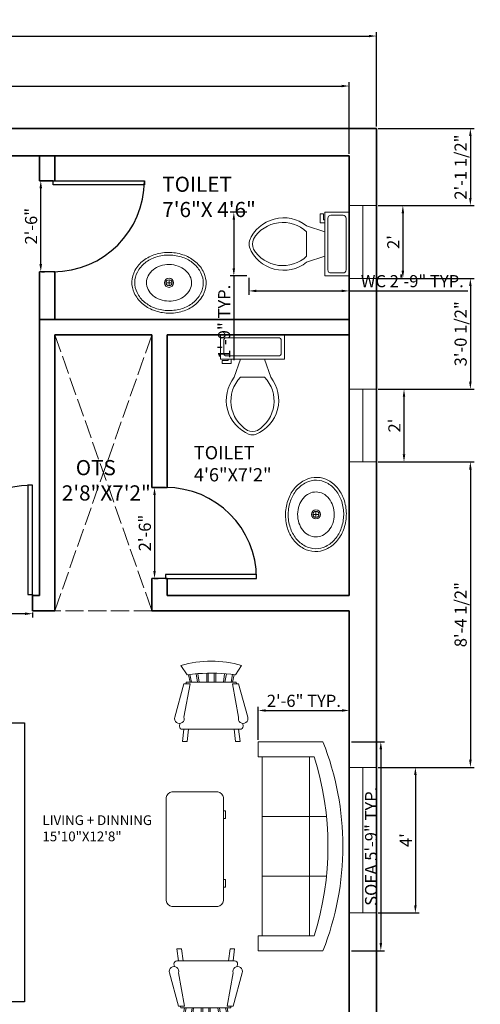
# Model space of a CAD drawing. Units: inches. Extents: x 2170 to 3011, y 1733 to 2338.
# Tile 3 of 5: x 2347 to 2498, y 2014 to 2338. Entities that reach past the tile are written whole.
import ezdxf

# ---------------------------------------------------------------- set-up
doc = ezdxf.new("R2010")
doc.units = ezdxf.units.IN
doc.linetypes.add('ACAD_ISO02W100', pattern=[15, 12, -3])
for name, color, linetype, lineweight in [('A-AREA-IDEN', 4, 'Continuous', 18), ('A-FLOR-FIXT', 20, 'Continuous', 18), ('A-FLOR-OPEN', 7, 'Continuous', 25), ('A-FLOR-OPEN-HIDN', 7, 'ACAD_ISO02W100', 13), ('A-WALL', 7, 'Continuous', 35), ('dim', 11, 'Continuous', 18), ('door', 6, 'Continuous', 25), ('furnitures', 20, 'Continuous', 18), ('window', 3, 'Continuous', 20)]:
    doc.layers.add(name, color=color, linetype=linetype, lineweight=lineweight)
doc.styles.get("Standard").update_dxf_attribs({"font": 'arial.ttf'})
doc.dimstyles.new('ISO-25', dxfattribs={"dimtxt": 4, "dimasz": 2.5, "dimexe": 1.25, "dimexo": 0.625, "dimtad": 1, "dimlunit": 3, "dimtxsty": 'Standard', "dimcen": 2.5, "dimadec": 0, "dimazin": 0, "dimtfac": 1, "dimtmove": 0, "dimatfit": 3, "dimfxl": 1, "dimarcsym": 0})

# ---------------------------------------------------------------- blocks, each defined once
blk = doc.blocks.new('*U3')
for p, q in [((0, 0), (0, -6)), ((-40, 0), (-40, -6))]:
    blk.add_line(p, q)
blk.add_lwpolyline([(0, 0), (0, 40), (-1.75, 40), (-1.75, 0)], close=True)
blk.add_arc((0, 0), 40, 90, 180)
blk = doc.blocks.new('*U2')
for p, q in [((0, 0), (0, -6)), ((40, 0), (40, -6))]:
    blk.add_line(p, q)
blk.add_lwpolyline([(0, 0), (0, 40), (1.75, 40), (1.75, 0)], close=True)
blk.add_arc((0, 0), 40, 0, 90)
blk = doc.blocks.new('Toilet - top')
for p, q in [((9.5, -6), (9.5, -2)), ((-10, -8.5), (-8, -8.5)), ((-10, -9.5), (-10, -8.5)), ((-7, -9.5), (-10, -9.5)), ((-8, -8.5), (-8, -8)), ((-7, -8), (-7, -9.5)), ((-4, -8), (-6, -14)), ((4, -8), (6, -14)), ((4, -14), (-4, -14))]:
    blk.add_line(p, q)
blk.add_lwpolyline([(10.5, -8), (10.5, 0), (-10.5, 0), (-10.5, -8)], close=True)
for points in [[(-9.5, -2), (-9.5, -6)], [(8.5, -1), (-8.5, -1)], [(-8.5, -7), (8.5, -7)]]:
    blk.add_lwpolyline(points)
for centre, radius, start, end in [((-8.62, -1.88), 0.884, 81.8699, 188.1301), ((8.62, -1.88), 0.884, 351.8699, 98.1301), ((-8.62, -6.12), 0.884, 171.8699, 278.1301), ((8.62, -6.12), 0.884, 261.8699, 8.1301), ((3.52, -21.58), 12.17, 141.4691, 247.9714), ((4.2, -21.82), 11.33, 136.3677, 238.9468), ((-3.52, -21.58), 12.17, 292.0284, 38.5307), ((-4.2, -21.82), 11.33, 301.053, 43.6321), ((0, -27.88), 4, 245.7318, 294.2682), ((0, -29), 4, 254.8605, 285.1395)]:
    blk.add_arc(centre, radius, start, end)
blk = doc.blocks.new('Sink - Oval top')
for p, q in [((-1, 0), (1, 0)), ((0, 1), (0, -1))]:
    blk.add_line(p, q)
for points in [[(-12.23, 0.39, 0.117634), (-11.46, -3.36, 0.104469), (-8.88, -6.8, 0.090016), (-5.08, -9.07, 0.08192), (-0.32, -10.02, 0.08192), (4.49, -9.38, 0.090016), (8.42, -7.36, 0.104469), (11.22, -4.09, 0.117634), (12.23, -0.39, 0.117634), (11.46, 3.36, 0.104469), (8.88, 6.8, 0.090016), (5.08, 9.07, 0.08192), (0.32, 10.02, 0.08192), (-4.49, 9.38, 0.090016), (-8.42, 7.36, 0.104469), (-11.22, 4.09, 0.117634)], [(-11.29, 0.16, 0.118622), (-10.52, -3.25, 0.104678), (-8.07, -6.36, 0.089562), (-4.54, -8.37, 0.081185), (-0.13, -9.15, 0.081185), (4.3, -8.49, 0.089562), (7.89, -6.58, 0.104678), (10.42, -3.55, 0.118622), (11.29, -0.16, 0.118622), (10.52, 3.25, 0.104678), (8.07, 6.36, 0.089562), (4.54, 8.37, 0.081185), (0.13, 9.15, 0.081185), (-4.3, 8.49, 0.089562), (-7.89, 6.58, 0.104678), (-10.42, 3.55, 0.118622)], [(-7.42, 0.08, 0.118283), (-6.91, -2.17, 0.104607), (-5.29, -4.21, 0.089718), (-2.97, -5.53, 0.081436), (-0.07, -6.04, 0.081436), (2.84, -5.59, 0.089718), (5.2, -4.33, 0.104607), (6.86, -2.32, 0.118283), (7.42, -0.08, 0.118283), (6.91, 2.17, 0.104607), (5.29, 4.21, 0.089718), (2.97, 5.53, 0.081436), (0.07, 6.04, 0.081436), (-2.84, 5.59, 0.089718), (-5.2, 4.33, 0.104607), (-6.86, 2.32, 0.118283)]]:
    blk.add_lwpolyline(points, format="xyb", close=True)
for radius in [1.5, 1]:
    blk.add_circle((0, 0), radius)
blk = doc.blocks.new('Desk - 30 x 60 in.')
for p, q in [((-26.999995, 0), (26.999995, 0)), ((-29.999995, -27), (-29.999995, -3)), ((29.999995, -3), (29.999995, -27)), ((26.999995, -30), (-26.999995, -30)), ((-20.000005, -30), (-20.000005, -31)), ((-16.000005, -31), (-16.000005, -30)), ((15.999995, -31), (15.999995, -30)), ((19.999995, -30), (19.999995, -31)), ((-20.000005, -31), (-16.000005, -31)), ((19.999995, -31), (15.999995, -31))]:
    blk.add_line(p, q)
for centre, start, end in [((-26.499995, -3.5), 98.1301, 171.8699), ((26.499995, -3.5), 8.130102, 81.8699), ((-26.499995, -26.5), 188.1301, 261.8699), ((26.499995, -26.5), 278.1301, 351.8699)]:
    blk.add_arc(centre, 3.535534, start, end)
blk = doc.blocks.new('Sofa - Roundback 7 ft.')
for p, q in [((-12.00002, -32.4421), (-12.00003, -6.5971)), ((11.99997, -32.4421), (11.99998, -6.5971)), ((-36.000027, -34), (-36.000027, -11.4696)), ((35.99998, -34), (35.99998, -11.4696)), ((-35.999844, -13.3819), (35.9998, -13.3819)), ((-36.000027, -32.4421), (35.99998, -32.4421))]:
    blk.add_line(p, q)
for points in [[(-36.000027, -34), (-42.000027, -34), (-42.000027, -8)], [(41.99998, -8), (41.99998, -34), (35.99998, -34)]]:
    blk.add_lwpolyline(points)
for centre, radius, start, end in [((0, -114.25), 114.25, 68.43141, 111.5686), ((-0.00001, -127.1968), 121.1968, 72.72033, 107.2797)]:
    blk.add_arc(centre, radius, start, end)
blk = doc.blocks.new('Chair - Rocking')
for p, q in [((-8, -4.5), (-10, -1.5)), ((8, -4.5), (10, -1.5)), ((-7.5, -4.5), (-7, -7)), ((-6.5, -7), (-7.02225, -4.43)), ((-4.5, -7), (-4.96674, -4.19951)), ((-4, -7), (-4.40532, -4.16272)), ((-1.5, -4.05012), (-1.5, -7)), ((-1, -7), (-1, -4.05012)), ((1, -7), (1, -4.04655)), ((1.5, -4.05012), (1.5, -7)), ((4, -7), (4.40187, -4.18694)), ((4.5, -7), (4.96761, -4.19437)), ((6.5, -7), (7, -4.4057)), ((7.5, -4.5), (7, -7)), ((-9, -7.5), (-12, -18.49999)), ((-7, -7.5), (-9, -7.5)), ((-9, -18.49999), (-7, -7.5)), ((-8.23428, -6.99939), (-8.3093, -7.47958)), ((-8.23041, -7), (8.23915, -7)), ((7, -7.5), (9, -7.5)), ((9, -18.49999), (7, -7.5)), ((8.31071, -7.48854), (8.23449, -7.00073)), ((9, -7.5), (12, -18.49999)), ((-10.36644, -20.64523), (-10.5, -21.49999)), ((-9, -22.49999), (-9.5, -26.49999)), ((0, -22.49999), (-9.5, -22.49999)), ((-8, -26.49999), (-7.5, -22.49999)), ((0, -22.49999), (9.5, -22.49999)), ((8, -26.49999), (7.5, -22.49999)), ((9, -22.49999), (9.5, -26.49999)), ((10.5, -21.49999), (10.3575, -20.58798)), ((-9.5, -26.49999), (-8, -26.49999)), ((9.5, -26.49999), (8, -26.49999))]:
    blk.add_line(p, q)
for centre, radius, start, end in [((0, -34.08333), 34.08333, 72.93847, 107.0615), ((0, -68.25004), 64.25, 93.92211, 97.15267), ((0, -68.25004), 64.25, 82.84733, 93.92211), ((-10.5, -18.99999), 1.58114, 161.5651, 18.43495), ((10.5, -18.99999), 1.58114, 161.5651, 18.43495), ((-9.5, -21.49999), 1, 180, 270), ((9.5, -21.49999), 1, 270, 0)]:
    blk.add_arc(centre, radius, start, end)
blk = doc.blocks.new('*D22')
at = {"layer": 'Defpoints', "color": 0, "transparency": 16777216}
for p in [(2455.17, 2316.33), (2215.17, 2293.31), (2455.17, 2293.31)]:
    blk.add_point(p, dxfattribs=at)
at = {"layer": 'dim', "color": 0, "lineweight": -2, "transparency": 16777216}
for p, q in [((2215.17, 2293.93), (2215.17, 2317.58)), ((2217.67, 2316.33), (2452.67, 2316.33)), ((2455.17, 2293.93), (2455.17, 2317.58))]:
    blk.add_line(p, q, dxfattribs=at)
at = {"layer": 'dim', "color": 0, "transparency": 16777216}
for points in [[(2217.67, 2316.74), (2217.67, 2315.91), (2215.17, 2316.33)], [(2452.67, 2316.74), (2452.67, 2315.91), (2455.17, 2316.33)]]:
    blk.add_solid(points, dxfattribs=at)
at = {"layer": 'dim', "color": 0, "transparency": 16777216, "insert": (2335.17, 2318.99), "char_height": 4, "attachment_point": 5}
blk.add_mtext("20'", dxfattribs=at)
blk = doc.blocks.new('*D24')
at = {"layer": 'Defpoints', "color": 0, "transparency": 16777216}
for p in [(2314.84, 2143.31), (2350.84, 2143.31), (2314.84, 2142.31)]:
    blk.add_point(p, dxfattribs=at)
at = {"layer": 'dim', "color": 0, "lineweight": -2, "transparency": 16777216}
for p, q in [((2314.84, 2142.68), (2314.84, 2141.06)), ((2348.34, 2142.31), (2317.34, 2142.31)), ((2350.84, 2142.68), (2350.84, 2141.06))]:
    blk.add_line(p, q, dxfattribs=at)
at = {"layer": 'dim', "color": 0, "transparency": 16777216}
for points in [[(2317.34, 2142.73), (2317.34, 2141.9), (2314.84, 2142.31)], [(2348.34, 2142.73), (2348.34, 2141.9), (2350.84, 2142.31)]]:
    blk.add_solid(points, dxfattribs=at)
at = {"layer": 'dim', "color": 0, "transparency": 16777216, "insert": (2332.84, 2144.98), "char_height": 4, "attachment_point": 5}
blk.add_mtext("3'", dxfattribs=at)
blk = doc.blocks.new('*D25')
at = {"layer": 'Defpoints', "color": 0, "transparency": 16777216}
for p in [(2390.17, 2183.93), (2390.17, 2153.93), (2391.03, 2153.93)]:
    blk.add_point(p, dxfattribs=at)
at = {"layer": 'dim', "color": 0, "lineweight": -2, "transparency": 16777216}
for p, q in [((2390.79, 2183.93), (2392.28, 2183.93)), ((2391.03, 2181.43), (2391.03, 2156.43)), ((2390.79, 2153.93), (2392.28, 2153.93))]:
    blk.add_line(p, q, dxfattribs=at)
at = {"layer": 'dim', "color": 0, "transparency": 16777216}
for points in [[(2390.61, 2181.43), (2391.45, 2181.43), (2391.03, 2183.93)], [(2390.61, 2156.43), (2391.45, 2156.43), (2391.03, 2153.93)]]:
    blk.add_solid(points, dxfattribs=at)
at = {"layer": 'dim', "color": 0, "transparency": 16777216, "insert": (2388.36, 2168.93), "char_height": 4, "attachment_point": 5, "rotation": 90}
blk.add_mtext('2\'-6"', dxfattribs=at)
blk = doc.blocks.new('*D26')
at = {"layer": 'Defpoints', "color": 0, "transparency": 16777216}
for p in [(2353.17, 2285.1), (2353.53, 2285.1), (2353.17, 2255.1)]:
    blk.add_point(p, dxfattribs=at)
at = {"layer": 'dim', "color": 0, "lineweight": -2, "transparency": 16777216}
for p, q in [((2353.53, 2257.6), (2353.53, 2282.6)), ((2353.79, 2285.1), (2354.78, 2285.1)), ((2353.79, 2255.1), (2354.78, 2255.1))]:
    blk.add_line(p, q, dxfattribs=at)
at = {"layer": 'dim', "color": 0, "transparency": 16777216}
for points in [[(2353.11, 2282.6), (2353.95, 2282.6), (2353.53, 2285.1)], [(2353.11, 2257.6), (2353.95, 2257.6), (2353.53, 2255.1)]]:
    blk.add_solid(points, dxfattribs=at)
at = {"layer": 'dim', "color": 0, "transparency": 16777216, "insert": (2350.86, 2270.1), "char_height": 4, "attachment_point": 5, "rotation": 90}
blk.add_mtext('2\'-6"', dxfattribs=at)
blk = doc.blocks.new('*D30')
at = {"layer": 'Defpoints', "color": 0, "transparency": 16777216}
for p in [(2464.17, 2091.66), (2464.17, 2043.66), (2477.01, 2043.66)]:
    blk.add_point(p, dxfattribs=at)
at = {"layer": 'dim', "color": 0, "lineweight": -2, "transparency": 16777216}
for p, q in [((2464.79, 2091.66), (2478.26, 2091.66)), ((2477.01, 2089.16), (2477.01, 2046.16)), ((2464.79, 2043.66), (2478.26, 2043.66))]:
    blk.add_line(p, q, dxfattribs=at)
at = {"layer": 'dim', "color": 0, "transparency": 16777216}
for points in [[(2476.6, 2089.16), (2477.43, 2089.16), (2477.01, 2091.66)], [(2476.6, 2046.16), (2477.43, 2046.16), (2477.01, 2043.66)]]:
    blk.add_solid(points, dxfattribs=at)
at = {"layer": 'dim', "color": 0, "transparency": 16777216, "insert": (2474.39, 2067.66), "char_height": 4, "attachment_point": 5, "rotation": 90}
blk.add_mtext("4'", dxfattribs=at)
blk = doc.blocks.new('*D31')
at = {"layer": 'Defpoints', "color": 0, "transparency": 16777216}
for p in [(2464.17, 2276.89), (2464.17, 2252.89), (2472.88, 2252.89)]:
    blk.add_point(p, dxfattribs=at)
at = {"layer": 'dim', "color": 0, "lineweight": -2, "transparency": 16777216}
for p, q in [((2464.79, 2276.89), (2474.13, 2276.89)), ((2472.88, 2274.39), (2472.88, 2255.39)), ((2464.79, 2252.89), (2474.13, 2252.89))]:
    blk.add_line(p, q, dxfattribs=at)
at = {"layer": 'dim', "color": 0, "transparency": 16777216}
for points in [[(2472.47, 2274.39), (2473.3, 2274.39), (2472.88, 2276.89)], [(2472.47, 2255.39), (2473.3, 2255.39), (2472.88, 2252.89)]]:
    blk.add_solid(points, dxfattribs=at)
at = {"layer": 'dim', "color": 0, "transparency": 16777216, "insert": (2470.25, 2264.89), "char_height": 4, "attachment_point": 5, "rotation": 90}
blk.add_mtext("2'", dxfattribs=at)
blk = doc.blocks.new('*D32')
at = {"layer": 'Defpoints', "color": 0, "transparency": 16777216}
for p in [(2464.17, 2216.36), (2473.26, 2216.36), (2464.17, 2192.36)]:
    blk.add_point(p, dxfattribs=at)
at = {"layer": 'dim', "color": 0, "lineweight": -2, "transparency": 16777216}
for p, q in [((2464.79, 2216.36), (2474.51, 2216.36)), ((2473.26, 2194.86), (2473.26, 2213.86)), ((2464.79, 2192.36), (2474.51, 2192.36))]:
    blk.add_line(p, q, dxfattribs=at)
at = {"layer": 'dim', "color": 0, "transparency": 16777216}
for points in [[(2472.84, 2213.86), (2473.67, 2213.86), (2473.26, 2216.36)], [(2472.84, 2194.86), (2473.67, 2194.86), (2473.26, 2192.36)]]:
    blk.add_solid(points, dxfattribs=at)
at = {"layer": 'dim', "color": 0, "transparency": 16777216, "insert": (2470.62, 2204.36), "char_height": 4, "attachment_point": 5, "rotation": 90}
blk.add_mtext("2'", dxfattribs=at)
blk = doc.blocks.new('WINDOW-48x9')
blk.add_line((4.5, 48), (4.5, 0))
blk.add_lwpolyline([(0, 48), (9, 48), (9, 0), (0, 0)], close=True)
blk = doc.blocks.new('WINDOW-24x9')
blk.add_line((4.5, 24), (4.5, 0))
blk.add_lwpolyline([(0, 24), (9, 24), (9, 0), (0, 0)], close=True)
blk = doc.blocks.new('*D54')
at = {"layer": 'Defpoints', "color": 0, "transparency": 16777216}
for p in [(2422.12, 2253.72), (2455.17, 2253.72), (2455.17, 2248.76)]:
    blk.add_point(p, dxfattribs=at)
at = {"layer": 'dim', "color": 0, "lineweight": -2, "transparency": 16777216}
for p, q in [((2422.12, 2253.09), (2422.12, 2247.51)), ((2455.17, 2253.09), (2455.17, 2247.51)), ((2424.62, 2248.76), (2452.67, 2248.76)), ((2455.17, 2248.76), (2494.33, 2248.76))]:
    blk.add_line(p, q, dxfattribs=at)
at = {"layer": 'dim', "color": 0, "transparency": 16777216}
for points in [[(2424.62, 2249.18), (2424.62, 2248.35), (2422.12, 2248.76)], [(2452.67, 2249.18), (2452.67, 2248.35), (2455.17, 2248.76)]]:
    blk.add_solid(points, dxfattribs=at)
at = {"layer": 'dim', "color": 0, "transparency": 16777216, "insert": (2476, 2251.46), "char_height": 4, "attachment_point": 5}
blk.add_mtext('WC 2\'-9" TYP.', dxfattribs=at)
blk = doc.blocks.new('*D55')
at = {"layer": 'Defpoints', "color": 0, "transparency": 16777216}
for p in [(2422.12, 2274.72), (2417.17, 2253.72), (2422.12, 2253.72)]:
    blk.add_point(p, dxfattribs=at)
at = {"layer": 'dim', "color": 0, "lineweight": -2, "transparency": 16777216}
for p, q in [((2421.5, 2274.72), (2415.92, 2274.72)), ((2417.17, 2272.22), (2417.17, 2256.22)), ((2421.5, 2253.72), (2415.92, 2253.72)), ((2417.17, 2253.72), (2417.17, 2225.96))]:
    blk.add_line(p, q, dxfattribs=at)
at = {"layer": 'dim', "color": 0, "transparency": 16777216}
for points in [[(2416.75, 2272.22), (2417.58, 2272.22), (2417.17, 2274.72)], [(2416.75, 2256.22), (2417.58, 2256.22), (2417.17, 2253.72)]]:
    blk.add_solid(points, dxfattribs=at)
at = {"layer": 'dim', "color": 0, "transparency": 16777216, "insert": (2414.5, 2238.59), "char_height": 4, "attachment_point": 5, "rotation": 90}
blk.add_mtext('1\'-9" TYP.', dxfattribs=at)
blk = doc.blocks.new('*D66')
at = {"layer": 'Defpoints', "color": 0, "transparency": 16777216}
for p in [(2455.29, 2100.07), (2455.29, 2031.18), (2465.62, 2031.18)]:
    blk.add_point(p, dxfattribs=at)
at = {"layer": 'dim', "color": 0, "lineweight": -2, "transparency": 16777216}
for p, q in [((2455.91, 2100.07), (2466.87, 2100.07)), ((2465.62, 2097.57), (2465.62, 2033.68)), ((2455.91, 2031.18), (2466.87, 2031.18))]:
    blk.add_line(p, q, dxfattribs=at)
at = {"layer": 'dim', "color": 0, "transparency": 16777216}
for points in [[(2465.2, 2097.57), (2466.04, 2097.57), (2465.62, 2100.07)], [(2465.2, 2033.68), (2466.04, 2033.68), (2465.62, 2031.18)]]:
    blk.add_solid(points, dxfattribs=at)
at = {"layer": 'dim', "color": 0, "transparency": 16777216, "insert": (2462.93, 2065.63), "char_height": 4, "attachment_point": 5, "rotation": 90}
blk.add_mtext('SOFA 5\'-9" TYP.', dxfattribs=at)
blk = doc.blocks.new('*D67')
at = {"layer": 'Defpoints', "color": 0, "transparency": 16777216}
for p in [(2455.29, 2110.41), (2425.21, 2100.07), (2455.29, 2100.07)]:
    blk.add_point(p, dxfattribs=at)
at = {"layer": 'dim', "color": 0, "lineweight": -2, "transparency": 16777216}
for p, q in [((2425.21, 2100.7), (2425.21, 2111.66)), ((2455.29, 2100.7), (2455.29, 2111.66)), ((2427.71, 2110.41), (2452.79, 2110.41))]:
    blk.add_line(p, q, dxfattribs=at)
at = {"layer": 'dim', "color": 0, "transparency": 16777216}
for points in [[(2427.71, 2110.82), (2427.71, 2109.99), (2425.21, 2110.41)], [(2452.79, 2110.82), (2452.79, 2109.99), (2455.29, 2110.41)]]:
    blk.add_solid(points, dxfattribs=at)
at = {"layer": 'dim', "color": 0, "transparency": 16777216, "insert": (2440.25, 2113.08), "char_height": 4, "attachment_point": 5}
blk.add_mtext('2\'-6" TYP.', dxfattribs=at)
blk = doc.blocks.new('*D85')
at = {"layer": 'Defpoints', "color": 0, "transparency": 16777216}
for p in [(2464.17, 2302.31), (2464.17, 2276.89), (2495.13, 2276.89)]:
    blk.add_point(p, dxfattribs=at)
at = {"layer": 'dim', "color": 0, "lineweight": -2, "transparency": 16777216}
for p, q in [((2464.79, 2302.31), (2496.38, 2302.31)), ((2495.13, 2299.81), (2495.13, 2279.39)), ((2464.79, 2276.89), (2496.38, 2276.89))]:
    blk.add_line(p, q, dxfattribs=at)
at = {"layer": 'dim', "color": 0, "transparency": 16777216}
for points in [[(2494.72, 2299.81), (2495.55, 2299.81), (2495.13, 2302.31)], [(2494.72, 2279.39), (2495.55, 2279.39), (2495.13, 2276.89)]]:
    blk.add_solid(points, dxfattribs=at)
at = {"layer": 'dim', "color": 0, "transparency": 16777216, "insert": (2492.44, 2289.6), "char_height": 4, "attachment_point": 5, "rotation": 90}
blk.add_mtext('2\'-1 1/2"', dxfattribs=at)
blk = doc.blocks.new('*D86')
at = {"layer": 'Defpoints', "color": 0, "transparency": 16777216}
for p in [(2464.17, 2252.89), (2464.17, 2216.36), (2495.13, 2216.36)]:
    blk.add_point(p, dxfattribs=at)
at = {"layer": 'dim', "color": 0, "lineweight": -2, "transparency": 16777216}
for p, q in [((2464.79, 2252.89), (2496.38, 2252.89)), ((2495.13, 2250.39), (2495.13, 2218.86)), ((2464.79, 2216.36), (2496.38, 2216.36))]:
    blk.add_line(p, q, dxfattribs=at)
at = {"layer": 'dim', "color": 0, "transparency": 16777216}
for points in [[(2494.72, 2250.39), (2495.55, 2250.39), (2495.13, 2252.89)], [(2494.72, 2218.86), (2495.55, 2218.86), (2495.13, 2216.36)]]:
    blk.add_solid(points, dxfattribs=at)
at = {"layer": 'dim', "color": 0, "transparency": 16777216, "insert": (2492.44, 2234.63), "char_height": 4, "attachment_point": 5, "rotation": 90}
blk.add_mtext('3\'-0 1/2"', dxfattribs=at)
blk = doc.blocks.new('*D87')
at = {"layer": 'Defpoints', "color": 0, "transparency": 16777216}
for p in [(2464.17, 2192.36), (2464.17, 2091.66), (2495.13, 2091.66)]:
    blk.add_point(p, dxfattribs=at)
at = {"layer": 'dim', "color": 0, "lineweight": -2, "transparency": 16777216}
for p, q in [((2464.79, 2192.36), (2496.38, 2192.36)), ((2495.13, 2189.86), (2495.13, 2094.16)), ((2464.79, 2091.66), (2496.38, 2091.66))]:
    blk.add_line(p, q, dxfattribs=at)
at = {"layer": 'dim', "color": 0, "transparency": 16777216}
for points in [[(2494.72, 2189.86), (2495.55, 2189.86), (2495.13, 2192.36)], [(2494.72, 2094.16), (2495.55, 2094.16), (2495.13, 2091.66)]]:
    blk.add_solid(points, dxfattribs=at)
at = {"layer": 'dim', "color": 0, "transparency": 16777216, "insert": (2492.44, 2142.01), "char_height": 4, "attachment_point": 5, "rotation": 90}
blk.add_mtext('8\'-4 1/2"', dxfattribs=at)
blk = doc.blocks.new('*D100')
at = {"layer": 'Defpoints', "color": 0, "transparency": 16777216}
for p in [(2464.17, 2332.81), (2206.17, 2302.31), (2464.17, 2302.31)]:
    blk.add_point(p, dxfattribs=at)
at = {"layer": 'dim', "color": 0, "lineweight": -2, "transparency": 16777216}
for p, q in [((2206.17, 2302.93), (2206.17, 2334.06)), ((2208.67, 2332.81), (2461.67, 2332.81)), ((2464.17, 2302.93), (2464.17, 2334.06))]:
    blk.add_line(p, q, dxfattribs=at)
at = {"layer": 'dim', "color": 0, "transparency": 16777216}
for points in [[(2208.67, 2333.22), (2208.67, 2332.39), (2206.17, 2332.81)], [(2461.67, 2333.22), (2461.67, 2332.39), (2464.17, 2332.81)]]:
    blk.add_solid(points, dxfattribs=at)
at = {"layer": 'dim', "color": 0, "transparency": 16777216, "insert": (2335.17, 2335.47), "char_height": 4, "attachment_point": 5}
blk.add_mtext('21\'-6"', dxfattribs=at)

msp = doc.modelspace()

# ---------------------------------------------------------------- linework, layer by layer
at = {"layer": 'A-FLOR-OPEN'}
msp.add_lwpolyline([(2252.169, 2106.306), (2348.169, 2106.306), (2348.169, 2014.306), (2252.169, 2014.306)], close=True, dxfattribs=at)
at = {"layer": 'A-FLOR-OPEN-HIDN', "ltscale": 0.5}
for p, q in [((2358.169, 2234.306), (2390.169, 2143.306)), ((2358.169, 2143.306), (2390.169, 2234.306)), ((2390.169, 2143.306), (2358.169, 2143.306))]:
    msp.add_line(p, q, dxfattribs=at)
at = {"layer": 'A-WALL'}
for p, q in [((2206.169, 2302.306), (2464.169, 2302.306)), ((2464.169, 1804.306), (2464.169, 2302.306)), ((2215.169, 2293.306), (2455.169, 2293.306)), ((2353.169, 2285.102), (2353.169, 2293.306)), ((2358.169, 2285.102), (2358.169, 2293.306)), ((2455.169, 2148.306), (2455.169, 2293.306)), ((2353.169, 2148.306), (2353.169, 2255.102)), ((2358.169, 2239.306), (2358.169, 2255.102)), ((2353.169, 2239.306), (2455.169, 2239.306)), ((2358.169, 2234.306), (2390.169, 2234.306)), ((2358.169, 2143.306), (2358.169, 2234.306)), ((2390.169, 2234.306), (2358.169, 2234.306)), ((2390.169, 2183.933), (2390.169, 2234.306)), ((2395.169, 2183.933), (2395.169, 2234.306)), ((2395.169, 2234.306), (2455.169, 2234.306)), ((2390.169, 2143.306), (2390.169, 2153.933)), ((2395.169, 2148.306), (2395.169, 2153.933)), ((2350.84, 2148.306), (2353.169, 2148.306)), ((2395.169, 2148.306), (2455.169, 2148.306)), ((2350.84, 2143.306), (2358.169, 2143.306)), ((2390.169, 2143.306), (2455.169, 2143.306)), ((2455.169, 1977.306), (2455.169, 2143.306))]:
    msp.add_line(p, q, dxfattribs=at)
msp.add_lwpolyline([(2350.84, 2148.306), (2350.84, 2143.306)], dxfattribs=at)
at = {"layer": 'door'}
for points in [[(2353.169, 2285.102), (2358.169, 2285.102)], [(2358.169, 2255.102), (2353.169, 2255.102)], [(2390.169, 2183.933), (2395.169, 2183.933)], [(2395.169, 2153.933), (2390.169, 2153.933)], [(2350.84, 2148.306), (2350.84, 2143.306)]]:
    msp.add_lwpolyline(points, dxfattribs=at)

# ---------------------------------------------------------------- block references
at = {"layer": 'A-FLOR-FIXT'}
for name, p, rotation in [('Toilet - top', (2455.169, 2264.219), 270.0000413745558), ('Sink - Oval top', (2444.227, 2175.052), 90)]:
    msp.add_blockref(name, p, dxfattribs=dict(at, rotation=rotation))
for name, p in [('Sink - Oval top', (2395.805, 2251.439)), ('Toilet - top', (2423.319, 2234.306))]:
    msp.add_blockref(name, p, dxfattribs=at)
at = {"layer": 'door', "xscale": 0.75, "yscale": 0.75, "zscale": 0.75, "rotation": 270}
for name, p in [('*U2', (2357.669, 2285.102)), ('*U3', (2394.669, 2153.933))]:
    msp.add_blockref(name, p, dxfattribs=at)
at = {"layer": 'door', "xscale": 0.9, "yscale": 0.9, "zscale": 0.9}
msp.add_blockref('*U3', (2350.84, 2148.706), dxfattribs=at)
at = {"layer": 'furnitures'}
msp.add_blockref('Chair - Rocking', (2409.738, 2126.708), dxfattribs=at)
for name, p, xscale, yscale, zscale, rotation in [('Sofa - Roundback 7 ft.', (2453.1, 2065.628), 0.820140253862633, 0.820140253862633, 0.820140253862633, 270), ('Desk - 30 x 60 in.', (2394.862, 2064.698), 0.6294377551275093, 0.6294377551275093, 0.6294377551275093, 90)]:
    msp.add_blockref(name, p, dxfattribs=dict(at, xscale=xscale, yscale=yscale, zscale=zscale, rotation=rotation))
at = {"layer": 'furnitures', "rotation": 180}
msp.add_blockref('Chair - Rocking', (2407.92, 2005.354), dxfattribs=at)
at = {"layer": 'window'}
for name, p in [('WINDOW-24x9', (2455.169, 2252.892)), ('WINDOW-24x9', (2455.169, 2192.363)), ('WINDOW-48x9', (2455.169, 2043.656))]:
    msp.add_blockref(name, p, dxfattribs=at)

# ---------------------------------------------------------------- texts
at = {"layer": 'A-AREA-IDEN', "attachment_point": 1}
for s, width, gutter_width, insert, char_height in [('TOILET\\P7\'6"X 4\'6"', 49.50568, 12.5, (2393.574, 2286.437), 5), ('TOILET\\P4\'6"X7\'2"', 43.24627, 10.92, (2404.003, 2197.594), 4.3678), ('   OTS\\P2\'8"X7\'2"', 49.50568, 12.5, (2360.479, 2192.985), 5), ('LIVING + DINNING\\P15\'10"X12\'8"', 42.80713, 8.019, (2354.091, 2075.836), 3.20762)]:
    msp.add_mtext_dynamic_manual_height_columns(s, width=width, gutter_width=gutter_width, heights=[0], dxfattribs=dict(at, insert=insert, char_height=char_height))

# ---------------------------------------------------------------- dimensions: what is measured, and where the dimension line sits
at = {"layer": 'dim'}
for base, p1, p2, override, picture, middle in [((2464.169, 2332.806), (2206.169, 2302.306), (2464.169, 2302.306), {"dimdec": 1, "dimlfac": 1, "dimrnd": 0, "dimzin": 1, "dimdsep": 46, "dimlunit": 4, "dimfrac": 2}, '*D100', (2335.169, 2335.474)), ((2455.169, 2316.325), (2215.169, 2293.306), (2455.169, 2293.306), {"dimclrd": 0, "dimclre": 0, "dimclrt": 0}, '*D22', (2335.169, 2318.992)), ((2314.84, 2142.315), (2350.84, 2143.306), (2314.84, 2143.306), {"dimclrd": 0, "dimclre": 0, "dimclrt": 0}, '*D24', (2332.84, 2144.984))]:
    dim = msp.add_linear_dim(base=base, p1=p1, p2=p2, dimstyle='ISO-25', override=override, dxfattribs=at)
    dim.commit()
    dim.dimension.update_dxf_attribs({"geometry": picture, "text_midpoint": middle})
for base, p1, p2, override, picture, middle in [((2495.135, 2276.892), (2464.169, 2302.306), (2464.169, 2276.892), {"dimdec": 1, "dimlfac": 1, "dimrnd": 0, "dimzin": 1, "dimdsep": 46, "dimlunit": 4, "dimfrac": 2}, '*D85', (2492.441, 2289.599)), ((2353.532, 2285.102), (2353.169, 2255.102), (2353.169, 2285.102), {"dimclrd": 0, "dimclre": 0, "dimclrt": 0}, '*D26', (2350.864, 2270.102)), ((2472.883, 2252.892), (2464.169, 2276.892), (2464.169, 2252.892), {"dimclrd": 0, "dimclre": 0, "dimclrt": 0}, '*D31', (2470.25, 2264.892)), ((2495.135, 2216.363), (2464.169, 2252.892), (2464.169, 2216.363), {"dimdec": 1, "dimlfac": 1, "dimrnd": 0, "dimzin": 1, "dimdsep": 46, "dimlunit": 4, "dimfrac": 2}, '*D86', (2492.44, 2234.627)), ((2473.257, 2216.363), (2464.169, 2192.363), (2464.169, 2216.363), {"dimclrd": 0, "dimclre": 0, "dimclrt": 0}, '*D32', (2470.623, 2204.363)), ((2495.135, 2091.656), (2464.169, 2192.363), (2464.169, 2091.656), {"dimdec": 1, "dimlfac": 1, "dimrnd": 0, "dimzin": 1, "dimdsep": 46, "dimlunit": 4, "dimfrac": 2}, '*D87', (2492.441, 2142.009)), ((2391.03, 2153.933), (2390.169, 2183.933), (2390.169, 2153.933), {"dimclrd": 0, "dimclre": 0, "dimclrt": 0}, '*D25', (2388.362, 2168.933)), ((2477.013, 2043.656), (2464.169, 2091.656), (2464.169, 2043.656), {"dimclrd": 0, "dimclre": 0, "dimclrt": 0}, '*D30', (2474.388, 2067.656))]:
    dim = msp.add_linear_dim(base=base, p1=p1, p2=p2, angle=90, dimstyle='ISO-25', override=override, dxfattribs=at)
    dim.commit()
    dim.dimension.update_dxf_attribs({"geometry": picture, "text_midpoint": middle})
for base, p1, p2, angle, text, picture, middle in [((2417.166, 2253.719), (2422.123, 2274.719), (2422.123, 2253.719), 270.00004, '<> TYP.', '*D55', (2414.499, 2238.591)), ((2455.169, 2248.762), (2422.123, 2253.719), (2455.169, 2253.719), 0.00004, 'WC <> TYP.', '*D54', (2475.998, 2251.455)), ((2465.62, 2031.182), (2455.287, 2100.074), (2455.287, 2031.182), 270, 'SOFA <> TYP.', '*D66', (2462.926, 2065.628))]:
    dim = msp.add_linear_dim(base=base, p1=p1, p2=p2, angle=angle, text=text, dimstyle='ISO-25', override={"dimdec": 1, "dimlfac": 1, "dimrnd": 0, "dimzin": 1, "dimdsep": 46, "dimlunit": 4, "dimfrac": 2}, dxfattribs=at)
    dim.commit()
    dim.dimension.update_dxf_attribs({"geometry": picture, "text_midpoint": middle})
dim = msp.add_linear_dim(base=(2455.287, 2110.408), p1=(2425.215, 2100.074), p2=(2455.287, 2100.074), text='<> TYP.', dimstyle='ISO-25', override={"dimdec": 1, "dimlfac": 1, "dimrnd": 0, "dimzin": 1, "dimdsep": 46, "dimlunit": 4, "dimfrac": 2}, dxfattribs=at)
dim.commit()
dim.dimension.update_dxf_attribs({"geometry": '*D67', "text_midpoint": (2440.251, 2113.075)})

doc.saveas('drawing.dxf')
